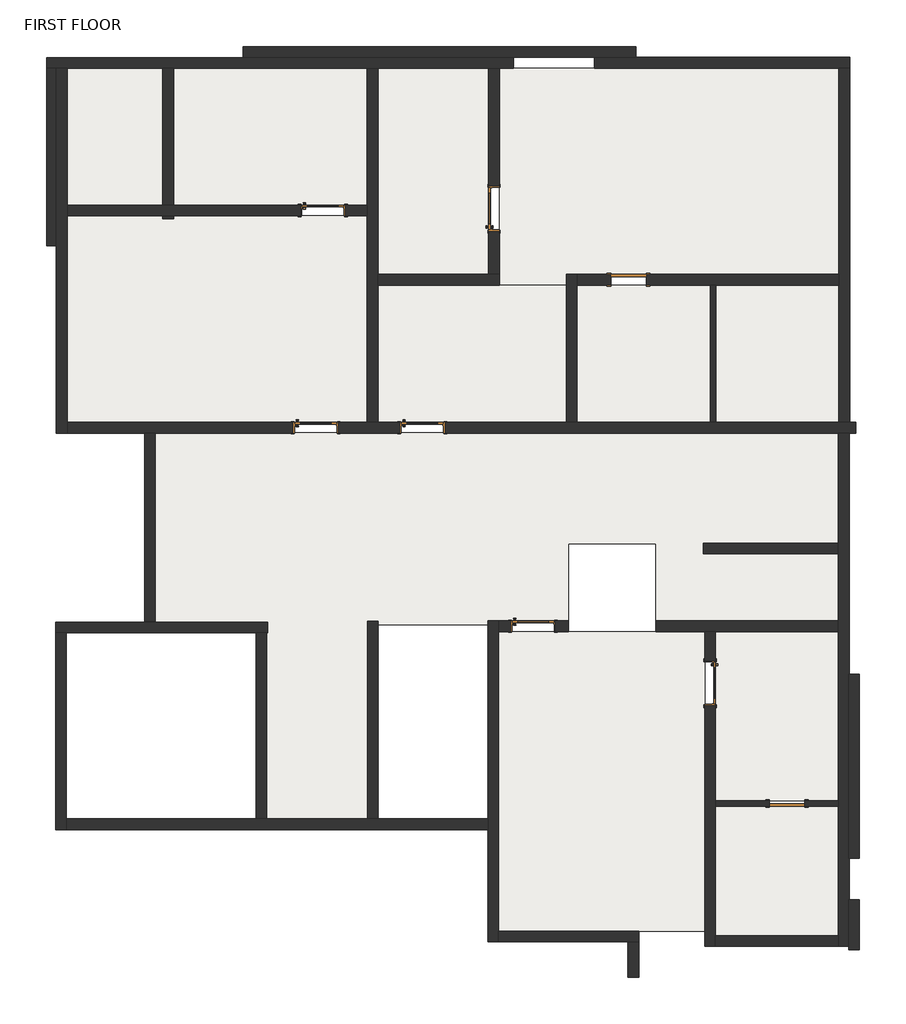
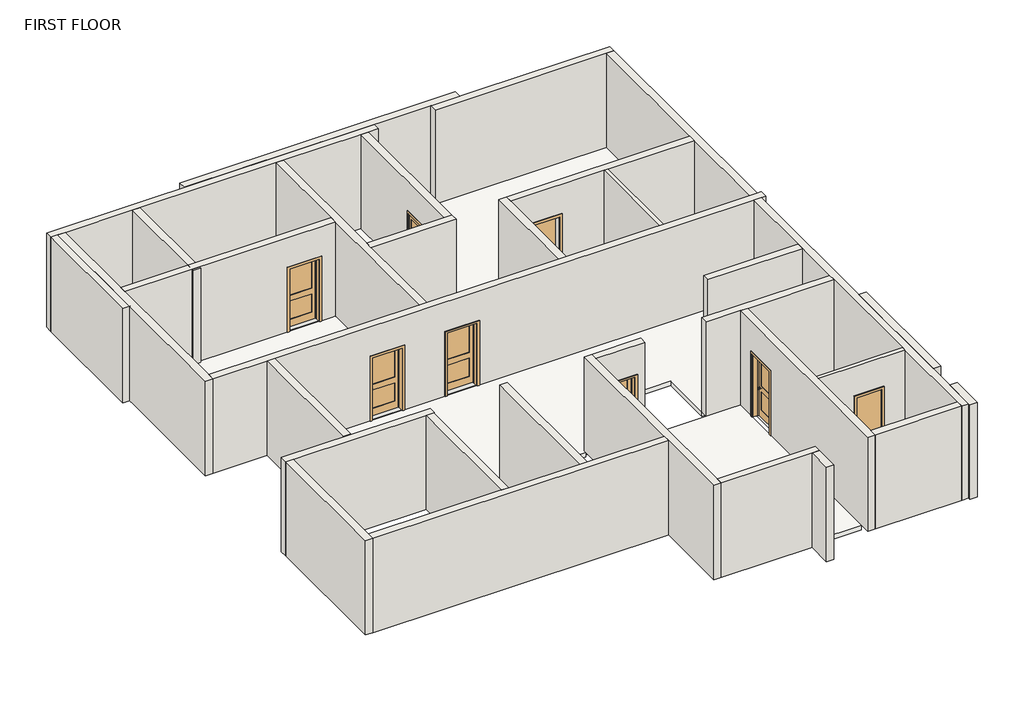
# One storey: 33 walls, 8 doors, 3 slabs.
"""IFC4 building model written with IfcOpenShell, lengths in millimetres."""

from ifc_helpers import new_model, si_unit, frame, origin, place, context, project, spatial, polyline, outline, extrude, faceted_brep, transform, mapped, element, save
from components import door_18b56f29, door_d8f5dbb5, door_a1484949

model = new_model("IFC4")

# Units and contexts
model_context = context("Model", 3, world=origin())
ifc_project = project(units=[si_unit("LENGTHUNIT", "METRE", prefix="MILLI")], contexts=[model_context])

# Site, building, storey
site = spatial("IfcSite", under=ifc_project)
building = spatial("IfcBuilding", under=site)
storey = spatial("IfcBuildingStorey", under=building, Name="FIRST FLOOR", Elevation=3048.0)

# Doors
placement = place(None, origin())
door_shape = door_18b56f29(model_context)
element("IfcDoor", 1, ObjectType="Door-Interior-Single-2_Panel-Wood : 36\" x 80\"", at=placement, inside=storey, context=model_context, shape_type="MappedRepresentation", body=[
    mapped(door_shape, transform((4633.8367729, 4367.107458, 3048.0), x_axis=(1.0, 0.0, 0.0), y_axis=(0.0, 1.0, 0.0), z_axis=(0.0, 0.0, 1.0))),
])
element("IfcDoor", 2, ObjectType="Door-Interior-Single-2_Panel-Wood : 36\" x 80\"", at=placement, inside=storey, context=model_context, shape_type="MappedRepresentation", body=[
    mapped(door_shape, transform((2258.0068953, 8623.6106247, 3048.0), x_axis=(1.0, 0.0, 0.0), y_axis=(0.0, 1.0, 0.0), z_axis=(0.0, 0.0, 1.0))),
])
element("IfcDoor", 3, ObjectType="Door-Interior-Single-2_Panel-Wood : 36\" x 80\"", at=placement, inside=storey, context=model_context, shape_type="MappedRepresentation", body=[
    mapped(door_shape, transform((-27.9931047, 8623.6106247, 3048.0), x_axis=(1.0, 0.0, 0.0), y_axis=(0.0, 1.0, 0.0), z_axis=(0.0, 0.0, 1.0))),
])
element("IfcDoor", 4, ObjectType="Door-Interior-Single-2_Panel-Wood : 36\" x 80\"", at=placement, inside=storey, context=model_context, shape_type="MappedRepresentation", body=[
    mapped(door_shape, transform((124.4068953, 13281.8847639, 3048.0), x_axis=(1.0, 0.0, 0.0), y_axis=(0.0, 1.0, 0.0), z_axis=(0.0, 0.0, 1.0))),
])
element("IfcDoor", 5, ObjectType="Door-Interior-Single-2_Panel-Wood : 36\" x 80\"", at=placement, inside=storey, context=model_context, shape_type="MappedRepresentation", body=[
    mapped(door_shape, transform((3792.558965, 13317.69348, 3048.0), x_axis=(0.0, 1.0, 0.0), y_axis=(-1.0, 0.0, 0.0), z_axis=(0.0, 0.0, 1.0))),
])
element("IfcDoor", 6, ObjectType="Door-Interior-Single-2_Panel-Wood : 36\" x 80\"", at=placement, inside=storey, context=model_context, shape_type="MappedRepresentation", body=[
    mapped(door_shape, transform((8433.5612453, 3144.732458, 3048.0), x_axis=(0.0, -1.0, 0.0), y_axis=(1.0, 0.0, 0.0), z_axis=(0.0, 0.0, 1.0))),
])
door_2_shape = door_d8f5dbb5(model_context)
element("IfcDoor", 7, ObjectType="Single-Flush : 30\" x 80\"", at=placement, inside=storey, context=model_context, shape_type="MappedRepresentation", body=[
    mapped(door_2_shape, transform((10080.5141504, 561.592156, 3048.0), x_axis=(-1.0, 0.0, 0.0), y_axis=(0.0, -1.0, 0.0), z_axis=(0.0, 0.0, 1.0))),
])
door_3_shape = door_a1484949(model_context)
element("IfcDoor", 8, ObjectType="Single-Flush : 30\" x 80\"", at=placement, inside=storey, context=model_context, shape_type="MappedRepresentation", body=[
    mapped(door_3_shape, transform((6680.3464182, 11793.69348, 3048.0), x_axis=(1.0, 0.0, 0.0), y_axis=(0.0, 1.0, 0.0), z_axis=(0.0, 0.0, 1.0))),
])

# Slabs
element("IfcSlab", 9, ObjectType="MARBLE FLOORING 6\"", at=placement, inside=storey, context=model_context, shape_type="SweptSolid", body=[
    extrude(outline(polyline([(-3306.644009, 16327.59348), (-3306.644009, 13393.0097639), (-5364.044009, 13393.0097639), (-5364.044009, 16327.59348), (-3306.644009, 16327.59348)])), frame((0.0, 0.0, 2895.6), z_axis=(0.0, 0.0, 1.0), x_axis=(1.0, 0.0, 0.0)), (0.0, 0.0, 1.0), 152.4),
    extrude(outline(polyline([(1076.9068953, 16327.59348), (1076.9068953, 13393.0097639), (-3078.044009, 13393.0097639), (-3078.044009, 16327.59348), (1076.9068953, 16327.59348)])), frame((0.0, 0.0, 2895.6), z_axis=(0.0, 0.0, 1.0), x_axis=(1.0, 0.0, 0.0)), (0.0, 0.0, 1.0), 152.4),
    extrude(outline(polyline([(3681.433965, 16327.59348), (3681.433965, 11907.99348), (1297.105991, 11907.99348), (1297.105991, 16327.59348), (3681.433965, 16327.59348)])), frame((0.0, 0.0, 2895.6), z_axis=(0.0, 0.0, 1.0), x_axis=(1.0, 0.0, 0.0)), (0.0, 0.0, 1.0), 152.4),
])
element("IfcSlab", 10, ObjectType="MARBLE FLOORING 6\"", at=placement, inside=storey, context=model_context, shape_type="SweptSolid", body=[
    extrude(outline(polyline([(1076.9068953, 13164.4097639), (1076.9068953, 8734.7356247), (-5364.044009, 8734.7356247), (-5364.044009, 13164.4097639), (1076.9068953, 13164.4097639)])), frame((0.0, 0.0, 2895.6), z_axis=(0.0, 0.0, 1.0), x_axis=(1.0, 0.0, 0.0)), (0.0, 0.0, 1.0), 152.4),
    extrude(outline(polyline([(5346.8464182, 11679.39348), (5346.8464182, 8734.7356247), (1305.5068953, 8734.7356247), (1305.5068953, 11679.39348), (5346.8464182, 11679.39348)])), frame((0.0, 0.0, 2895.6), z_axis=(0.0, 0.0, 1.0), x_axis=(1.0, 0.0, 0.0)), (0.0, 0.0, 1.0), 152.4),
])
element("IfcSlab", 11, ObjectType="MARBLE FLOORING 6\"", at=placement, inside=storey, context=model_context, shape_type="SweptSolid", body=[
    extrude(outline(polyline([(8440.081677, 11679.39348), (8440.081677, 8737.3195632), (5575.4464182, 8737.3195632), (5575.4464182, 11679.39348), (8440.081677, 11679.39348)])), frame((0.0, 0.0, 2895.6), z_axis=(0.0, 0.0, 1.0), x_axis=(1.0, 0.0, 0.0)), (0.0, 0.0, 1.0), 152.4),
    extrude(outline(polyline([(11195.981677, 11679.39348), (11195.981677, 8734.7356247), (8554.381677, 8734.7356247), (8554.381677, 11679.39348), (11195.981677, 11679.39348)])), frame((0.0, 0.0, 2895.6), z_axis=(0.0, 0.0, 1.0), x_axis=(1.0, 0.0, 0.0)), (0.0, 0.0, 1.0), 152.4),
    extrude(outline(polyline([(3910.033965, 11679.39348), (3910.033965, 16330.2375339), (11195.981677, 16330.2375339), (11195.981677, 11907.99348), (5346.8464182, 11907.99348), (5346.8464182, 11679.39348), (3910.033965, 11679.39348)])), frame((0.0, 0.0, 2895.6), z_axis=(0.0, 0.0, 1.0), x_axis=(1.0, 0.0, 0.0)), (0.0, 0.0, 1.0), 152.4),
    extrude(outline(polyline([(-3471.744009, 4450.8216143), (-3471.744009, 8508.7195632), (11198.9862453, 8508.7195632), (11198.9862453, 6146.76982), (8289.8141504, 6146.76982), (8289.8141504, 5918.16982), (11185.4141504, 5918.16982), (11185.4141504, 4478.232458), (7273.8141504, 4478.232458), (7273.8141504, 6129.232458), (5395.8367729, 6129.232458), (5395.8367729, 4478.232458), (3668.6367729, 4478.232458), (3668.6367729, 4400.0216143), (1309.2237558, 4400.0216143), (1309.2237558, 4476.2216143), (1080.6237558, 4476.2216143), (1080.6237558, 234.4216143), (-1082.0931047, 234.4216143), (-1082.0931047, 4222.2216143), (-1059.3262442, 4222.2216143), (-1059.3262442, 4450.8216143), (-3471.744009, 4450.8216143)])), frame((0.0, 0.0, 2895.6), z_axis=(0.0, 0.0, 1.0), x_axis=(1.0, 0.0, 0.0)), (0.0, 0.0, 1.0), 152.4),
    extrude(outline(polyline([(8316.0862453, -2170.217542), (3897.2367729, -2170.217542), (3897.2367729, 4249.632458), (8316.0862453, 4249.632458), (8316.0862453, -2170.217542)])), frame((0.0, 0.0, 2895.6), z_axis=(0.0, 0.0, 1.0), x_axis=(1.0, 0.0, 0.0)), (0.0, 0.0, 1.0), 152.4),
    extrude(outline(polyline([(8544.6862453, 618.742156), (8544.6862453, 4249.632458), (11185.4141504, 4249.632458), (11185.4141504, 618.742156), (8544.6862453, 618.742156)])), frame((0.0, 0.0, 2895.6), z_axis=(0.0, 0.0, 1.0), x_axis=(1.0, 0.0, 0.0)), (0.0, 0.0, 1.0), 152.4),
    extrude(outline(polyline([(8544.6862453, -2271.817542), (8544.6862453, 504.442156), (11185.4141504, 504.442156), (11185.4141504, -2271.817542), (8544.6862453, -2271.817542)])), frame((0.0, 0.0, 2895.6), z_axis=(0.0, 0.0, 1.0), x_axis=(1.0, 0.0, 0.0)), (0.0, 0.0, 1.0), 152.4),
])

# Walls
element("IfcWall", 12, ObjectType="INNER WALL 4.5\"", at=placement, inside=storey, context=model_context, shape_type="SweptSolid", body=[
    extrude(outline(polyline([(3048.0, 8544.6862453), (3048.0, 9699.5141504), (5080.0, 9699.5141504), (5080.0, 10461.5141504), (3048.0, 10461.5141504), (3048.0, 11185.4141504), (6096.0, 11185.4141504), (6096.0, 8544.6862453), (3048.0, 8544.6862453)])), frame((0.0, 504.442156, 0.0), z_axis=(0.0, 1.0, 0.0), x_axis=(0.0, 0.0, 1.0)), (0.0, 0.0, 1.0), 114.3),
])
element("IfcWall", 13, ObjectType="INNER WALL 4.5\"", at=placement, inside=storey, context=model_context, shape_type="SweptSolid", body=[
    extrude(outline(polyline([(8440.081677, 8737.3195632), (8440.081677, 11679.39348), (8554.381677, 11679.39348), (8554.381677, 8737.3195632), (8440.081677, 8737.3195632)])), frame((0.0, 0.0, 3048.0), z_axis=(0.0, 0.0, 1.0), x_axis=(1.0, 0.0, 0.0)), (0.0, 0.0, 1.0), 3048.0),
])
element("IfcWall", 14, ObjectType="OUTER WALL THICKNESS 9\"", at=placement, inside=storey, context=model_context, shape_type="Brep", body=[
    faceted_brep([(11424.581677, 16558.8375339, 3048.0), (5950.881677, 16558.8375339, 3048.0), (5950.881677, 16558.8375339, 6096.0), (11424.581677, 16558.8375339, 6096.0), (11424.581677, 16330.2375339, 3048.0), (11424.581677, 16330.2375339, 6096.0), (11195.981677, 16330.2375339, 6096.0), (5950.881677, 16330.2375339, 6096.0), (5950.881677, 16330.2375339, 3048.0), (11195.981677, 16330.2375339, 3048.0)], [[[0, 1, 2, 3]], [[4, 5, 6, 7, 8, 9]], [[1, 0, 4, 9, 8]], [[2, 1, 8, 7]], [[3, 2, 7, 6, 5]], [[0, 3, 5, 4]]]),
])
element("IfcWall", 15, ObjectType="OUTER WALL THICKNESS 9\"", at=placement, inside=storey, context=model_context, shape_type="SweptSolid", body=[
    extrude(outline(polyline([(-1588.9187543, 16792.7871664), (6843.8812457, 16792.7871664), (6843.8812457, 16564.1871664), (-1588.9187543, 16564.1871664), (-1588.9187543, 16792.7871664)])), frame((0.0, 0.0, 3048.0), z_axis=(0.0, 0.0, 1.0), x_axis=(1.0, 0.0, 0.0)), (0.0, 0.0, 1.0), 3048.0),
])
element("IfcWall", 16, ObjectType="OUTER WALL THICKNESS 9\"", at=placement, inside=storey, context=model_context, shape_type="Brep", body=[
    faceted_brep([(4217.331677, 16556.19348, 3048.0), (-5802.968323, 16556.19348, 3048.0), (-5802.968323, 16556.19348, 6096.0), (4217.331677, 16556.19348, 6096.0), (4217.331677, 16327.59348, 3048.0), (4217.331677, 16327.59348, 6096.0), (3910.033965, 16327.59348, 6096.0), (3681.433965, 16327.59348, 6096.0), (1305.5068953, 16327.59348, 6096.0), (1076.9068953, 16327.59348, 6096.0), (-3078.044009, 16327.59348, 6096.0), (-3306.644009, 16327.59348, 6096.0), (-5364.044009, 16327.59348, 6096.0), (-5574.368323, 16327.59348, 6096.0), (-5592.644009, 16327.59348, 6096.0), (-5802.968323, 16327.59348, 6096.0), (-5802.968323, 16327.59348, 3048.0), (-5592.644009, 16327.59348, 3048.0), (-5574.368323, 16327.59348, 3048.0), (-5364.044009, 16327.59348, 3048.0), (-3306.644009, 16327.59348, 3048.0), (-3078.044009, 16327.59348, 3048.0), (1076.9068953, 16327.59348, 3048.0), (1305.5068953, 16327.59348, 3048.0), (3681.433965, 16327.59348, 3048.0), (3910.033965, 16327.59348, 3048.0)], [[[0, 1, 2, 3]], [[4, 5, 6, 7, 8, 9, 10, 11, 12, 13, 14, 15, 16, 17, 18, 19, 20, 21, 22, 23, 24, 25]], [[1, 0, 4, 25, 24, 23, 22, 21, 20, 19, 18, 17, 16]], [[3, 2, 15, 14, 13, 12, 11, 10, 9, 8, 7, 6, 5]], [[0, 3, 5, 4]], [[2, 1, 16, 15]]]),
])
element("IfcWall", 17, ObjectType="OUTER WALL THICKNESS 9\"", at=placement, inside=storey, context=model_context, shape_type="SweptSolid", body=[
    extrude(outline(polyline([(-5802.968323, 12517.59348), (-5802.968323, 16327.59348), (-5574.368323, 16327.59348), (-5574.368323, 12517.59348), (-5802.968323, 12517.59348)])), frame((0.0, 0.0, 3048.0), z_axis=(0.0, 0.0, 1.0), x_axis=(1.0, 0.0, 0.0)), (0.0, 0.0, 1.0), 3048.0),
])
element("IfcWall", 18, ObjectType="OUTER WALL THICKNESS 9\"", at=placement, inside=storey, context=model_context, shape_type="Brep", body=[
    faceted_brep([(-5364.044009, 8504.39348, 3048.0), (-5364.044009, 8506.1356247, 3048.0), (-5364.044009, 8734.7356247, 3048.0), (-5364.044009, 13164.4097639, 3048.0), (-5364.044009, 13393.0097639, 3048.0), (-5364.044009, 16327.59348, 3048.0), (-5364.044009, 16327.59348, 6096.0), (-5364.044009, 13393.0097639, 6096.0), (-5364.044009, 13164.4097639, 6096.0), (-5364.044009, 8734.7356247, 6096.0), (-5364.044009, 8506.1356247, 6096.0), (-5364.044009, 8504.39348, 6096.0), (-5592.644009, 8504.39348, 3048.0), (-5592.644009, 8504.39348, 6096.0), (-5592.644009, 16327.59348, 6096.0), (-5592.644009, 16327.59348, 3048.0)], [[[0, 1, 2, 3, 4, 5, 6, 7, 8, 9, 10, 11]], [[12, 13, 14, 15]], [[5, 4, 3, 2, 1, 0, 12, 15]], [[11, 10, 9, 8, 7, 6, 14, 13]], [[0, 11, 13, 12]], [[6, 5, 15, 14]]]),
])
element("IfcWall", 19, ObjectType="OUTER WALL THICKNESS 9\"", at=placement, inside=storey, context=model_context, shape_type="Brep", body=[
    faceted_brep([(11552.355991, 8506.1356247, 3048.0), (11552.355991, 8506.1356247, 6096.0), (11414.0141504, 8506.1356247, 6096.0), (11185.4141504, 8506.1356247, 6096.0), (-5364.044009, 8506.1356247, 6096.0), (-5364.044009, 8506.1356247, 3048.0), (-510.5931047, 8506.1356247, 3048.0), (-510.5931047, 8506.1356247, 5105.4), (454.6068953, 8506.1356247, 5105.4), (454.6068953, 8506.1356247, 3048.0), (1775.4068953, 8506.1356247, 3048.0), (1775.4068953, 8506.1356247, 5105.4), (2740.6068953, 8506.1356247, 5105.4), (2740.6068953, 8506.1356247, 3048.0), (11185.4141504, 8506.1356247, 3048.0), (11414.0141504, 8506.1356247, 3048.0), (11552.355991, 8734.7356247, 6096.0), (11552.355991, 8734.7356247, 3048.0), (11424.581677, 8734.7356247, 3048.0), (11195.981677, 8734.7356247, 3048.0), (5575.4464182, 8734.7356247, 3048.0), (5346.8464182, 8734.7356247, 3048.0), (2740.6068953, 8734.7356247, 3048.0), (2740.6068953, 8734.7356247, 5105.4), (1775.4068953, 8734.7356247, 5105.4), (1775.4068953, 8734.7356247, 3048.0), (1305.5068953, 8734.7356247, 3048.0), (1076.9068953, 8734.7356247, 3048.0), (454.6068953, 8734.7356247, 3048.0), (454.6068953, 8734.7356247, 5105.4), (-510.5931047, 8734.7356247, 5105.4), (-510.5931047, 8734.7356247, 3048.0), (-5364.044009, 8734.7356247, 3048.0), (-5364.044009, 8734.7356247, 6096.0), (1076.9068953, 8734.7356247, 6096.0), (1305.5068953, 8734.7356247, 6096.0), (5346.8464182, 8734.7356247, 6096.0), (5575.4464182, 8734.7356247, 6096.0), (11195.981677, 8734.7356247, 6096.0), (11424.581677, 8734.7356247, 6096.0)], [[[0, 1, 2, 3, 4, 5, 6, 7, 8, 9, 10, 11, 12, 13, 14, 15]], [[16, 17, 18, 19, 20, 21, 22, 23, 24, 25, 26, 27, 28, 29, 30, 31, 32, 33, 34, 35, 36, 37, 38, 39]], [[17, 0, 15, 14, 13, 22, 21, 20, 19, 18]], [[5, 32, 31, 6]], [[25, 10, 9, 28, 27, 26]], [[1, 0, 17, 16]], [[4, 3, 2, 1, 16, 39, 38, 37, 36, 35, 34, 33]], [[5, 4, 33, 32]], [[12, 23, 22, 13]], [[23, 12, 11, 24]], [[24, 11, 10, 25]], [[8, 29, 28, 9]], [[29, 8, 7, 30]], [[30, 7, 6, 31]]]),
])
element("IfcWall", 20, ObjectType="OUTER WALL THICKNESS 9\"", at=placement, inside=storey, context=model_context, shape_type="Brep", body=[
    faceted_brep([(5575.4464182, 8734.7356247, 3048.0), (5575.4464182, 11679.39348, 3048.0), (5575.4464182, 11907.99348, 3048.0), (5575.4464182, 11907.99348, 6096.0), (5575.4464182, 11679.39348, 6096.0), (5575.4464182, 8734.7356247, 6096.0), (5346.8464182, 8734.7356247, 3048.0), (5346.8464182, 8734.7356247, 6096.0), (5346.8464182, 11907.99348, 6096.0), (5346.8464182, 11907.99348, 3048.0)], [[[0, 1, 2, 3, 4, 5]], [[6, 7, 8, 9]], [[2, 1, 0, 6, 9]], [[5, 4, 3, 8, 7]], [[0, 5, 7, 6]], [[3, 2, 9, 8]]]),
])
element("IfcWall", 21, ObjectType="OUTER WALL THICKNESS 9\"", at=placement, inside=storey, context=model_context, shape_type="Brep", body=[
    faceted_brep([(1305.5068953, 8734.7356247, 3048.0), (1305.5068953, 11679.39348, 3048.0), (1305.5068953, 11907.99348, 3048.0), (1305.5068953, 16327.59348, 3048.0), (1305.5068953, 16327.59348, 6096.0), (1305.5068953, 11907.99348, 6096.0), (1305.5068953, 11679.39348, 6096.0), (1305.5068953, 8734.7356247, 6096.0), (1076.9068953, 8734.7356247, 3048.0), (1076.9068953, 8734.7356247, 6096.0), (1076.9068953, 13164.4097639, 6096.0), (1076.9068953, 13393.0097639, 6096.0), (1076.9068953, 16327.59348, 6096.0), (1076.9068953, 16327.59348, 3048.0), (1076.9068953, 13393.0097639, 3048.0), (1076.9068953, 13164.4097639, 3048.0)], [[[0, 1, 2, 3, 4, 5, 6, 7]], [[8, 9, 10, 11, 12, 13, 14, 15]], [[3, 2, 1, 0, 8, 15, 14, 13]], [[7, 6, 5, 4, 12, 11, 10, 9]], [[4, 3, 13, 12]], [[0, 7, 9, 8]]]),
])
element("IfcWall", 22, ObjectType="OUTER WALL THICKNESS 9\"", at=placement, inside=storey, context=model_context, shape_type="SweptSolid", body=[
    extrude(outline(polyline([(-3306.644009, 13101.79348), (-3306.644009, 16327.59348), (-3078.044009, 16327.59348), (-3078.044009, 13101.79348), (-3306.644009, 13101.79348)])), frame((0.0, 0.0, 3048.0), z_axis=(0.0, 0.0, 1.0), x_axis=(1.0, 0.0, 0.0)), (0.0, 0.0, 1.0), 3048.0),
])
element("IfcWall", 23, ObjectType="OUTER WALL THICKNESS 9\"", at=placement, inside=storey, context=model_context, shape_type="SweptSolid", body=[
    extrude(outline(polyline([(6096.0, 1076.9068953), (6096.0, -5364.044009), (3048.0, -5364.044009), (3048.0, -358.1931047), (5105.4, -358.1931047), (5105.4, 607.0068953), (3048.0, 607.0068953), (3048.0, 1076.9068953), (6096.0, 1076.9068953)])), frame((0.0, 13164.4097639, 0.0), z_axis=(0.0, 1.0, 0.0), x_axis=(0.0, 0.0, 1.0)), (0.0, 0.0, 1.0), 228.6),
])
element("IfcWall", 24, ObjectType="OUTER WALL THICKNESS 9\"", at=placement, inside=storey, context=model_context, shape_type="Brep", body=[
    faceted_brep([(1305.5068953, 11679.39348, 3048.0), (3910.033965, 11679.39348, 3048.0), (3910.033965, 11679.39348, 6096.0), (1305.5068953, 11679.39348, 6096.0), (1305.5068953, 11907.99348, 3048.0), (1305.5068953, 11907.99348, 6096.0), (3681.433965, 11907.99348, 6096.0), (3910.033965, 11907.99348, 6096.0), (3910.033965, 11907.99348, 3048.0), (3681.433965, 11907.99348, 3048.0)], [[[0, 1, 2, 3]], [[4, 5, 6, 7, 8, 9]], [[1, 0, 4, 9, 8]], [[3, 2, 7, 6, 5]], [[0, 3, 5, 4]], [[2, 1, 8, 7]]]),
])
element("IfcWall", 25, ObjectType="OUTER WALL THICKNESS 9\"", at=placement, inside=storey, context=model_context, shape_type="SweptSolid", body=[
    extrude(outline(polyline([(11907.99348, 6096.0), (16327.59348, 6096.0), (16327.59348, 3048.0), (13800.29348, 3048.0), (13800.29348, 5105.4), (12835.09348, 5105.4), (12835.09348, 3048.0), (11907.99348, 3048.0), (11907.99348, 6096.0)])), frame((3681.433965, 0.0, 0.0), z_axis=(1.0, 0.0, 0.0), x_axis=(0.0, 1.0, 0.0)), (0.0, 0.0, 1.0), 228.6),
])
element("IfcWall", 26, ObjectType="OUTER WALL THICKNESS 9\"", at=placement, inside=storey, context=model_context, shape_type="Brep", body=[
    faceted_brep([(11414.0141504, -2500.417542, 3048.0), (11414.0141504, 8506.1356247, 3048.0), (11414.0141504, 8506.1356247, 6096.0), (11414.0141504, -2500.417542, 6096.0), (11185.4141504, -2500.417542, 3048.0), (11185.4141504, -2500.417542, 6096.0), (11185.4141504, -2271.817542, 6096.0), (11185.4141504, 504.442156, 6096.0), (11185.4141504, 618.742156, 6096.0), (11185.4141504, 4249.632458, 6096.0), (11185.4141504, 4478.232458, 6096.0), (11185.4141504, 5918.16982, 6096.0), (11185.4141504, 6146.76982, 6096.0), (11185.4141504, 8506.1356247, 6096.0), (11185.4141504, 8506.1356247, 3048.0), (11185.4141504, 6146.76982, 3048.0), (11185.4141504, 5918.16982, 3048.0), (11185.4141504, 4478.232458, 3048.0), (11185.4141504, 4249.632458, 3048.0), (11185.4141504, 618.742156, 3048.0), (11185.4141504, 504.442156, 3048.0), (11185.4141504, -2271.817542, 3048.0)], [[[0, 1, 2, 3]], [[4, 5, 6, 7, 8, 9, 10, 11, 12, 13, 14, 15, 16, 17, 18, 19, 20, 21]], [[1, 0, 4, 21, 20, 19, 18, 17, 16, 15, 14]], [[3, 2, 13, 12, 11, 10, 9, 8, 7, 6, 5]], [[2, 1, 14, 13]], [[0, 3, 5, 4]]]),
])
element("IfcWall", 27, ObjectType="OUTER WALL THICKNESS 9\"", at=placement, inside=storey, context=model_context, shape_type="Brep", body=[
    faceted_brep([(-5605.9262442, 4222.2216143, 3048.0), (-5377.3262442, 4222.2216143, 3048.0), (-1310.6931047, 4222.2216143, 3048.0), (-1082.0931047, 4222.2216143, 3048.0), (-1059.3262442, 4222.2216143, 3048.0), (-1059.3262442, 4222.2216143, 6096.0), (-1082.0931047, 4222.2216143, 6096.0), (-1310.6931047, 4222.2216143, 6096.0), (-5377.3262442, 4222.2216143, 6096.0), (-5605.9262442, 4222.2216143, 6096.0), (-5605.9262442, 4450.8216143, 3048.0), (-5605.9262442, 4450.8216143, 6096.0), (-1059.3262442, 4450.8216143, 6096.0), (-1059.3262442, 4450.8216143, 3048.0)], [[[0, 1, 2, 3, 4, 5, 6, 7, 8, 9]], [[10, 11, 12, 13]], [[4, 3, 2, 1, 0, 10, 13]], [[5, 4, 13, 12]], [[9, 8, 7, 6, 5, 12, 11]], [[0, 9, 11, 10]]]),
])
element("IfcWall", 28, ObjectType="OUTER WALL THICKNESS 9\"", at=placement, inside=storey, context=model_context, shape_type="SweptSolid", body=[
    extrude(outline(polyline([(-3700.344009, 4476.2216143), (-3700.344009, 8504.39348), (-3471.744009, 8504.39348), (-3471.744009, 4476.2216143), (-3700.344009, 4476.2216143)])), frame((0.0, 0.0, 3048.0), z_axis=(0.0, 0.0, 1.0), x_axis=(1.0, 0.0, 0.0)), (0.0, 0.0, 1.0), 3048.0),
])
element("IfcWall", 29, ObjectType="OUTER WALL THICKNESS 9\"", at=placement, inside=storey, context=model_context, shape_type="Brep", body=[
    faceted_brep([(-5605.9262442, 4222.2216143, 3048.0), (-5605.9262442, 5.8216143, 3048.0), (-5605.9262442, 5.8216143, 6096.0), (-5605.9262442, 4222.2216143, 6096.0), (-5377.3262442, 4222.2216143, 3048.0), (-5377.3262442, 4222.2216143, 6096.0), (-5377.3262442, 234.4216143, 6096.0), (-5377.3262442, 5.8216143, 6096.0), (-5377.3262442, 5.8216143, 3048.0), (-5377.3262442, 234.4216143, 3048.0)], [[[0, 1, 2, 3]], [[4, 5, 6, 7, 8, 9]], [[1, 0, 4, 9, 8]], [[3, 2, 7, 6, 5]], [[0, 3, 5, 4]], [[2, 1, 8, 7]]]),
])
element("IfcWall", 30, ObjectType="OUTER WALL THICKNESS 9\"", at=placement, inside=storey, context=model_context, shape_type="Brep", body=[
    faceted_brep([(3668.6367729, 234.4216143, 3048.0), (1309.2237558, 234.4216143, 3048.0), (1080.6237558, 234.4216143, 3048.0), (-1082.0931047, 234.4216143, 3048.0), (-1310.6931047, 234.4216143, 3048.0), (-5377.3262442, 234.4216143, 3048.0), (-5377.3262442, 234.4216143, 6096.0), (-1310.6931047, 234.4216143, 6096.0), (-1082.0931047, 234.4216143, 6096.0), (1080.6237558, 234.4216143, 6096.0), (1309.2237558, 234.4216143, 6096.0), (3668.6367729, 234.4216143, 6096.0), (3668.6367729, 5.8216143, 3048.0), (3668.6367729, 5.8216143, 6096.0), (-5377.3262442, 5.8216143, 6096.0), (-5377.3262442, 5.8216143, 3048.0)], [[[0, 1, 2, 3, 4, 5, 6, 7, 8, 9, 10, 11]], [[12, 13, 14, 15]], [[5, 4, 3, 2, 1, 0, 12, 15]], [[11, 10, 9, 8, 7, 6, 14, 13]], [[6, 5, 15, 14]], [[0, 11, 13, 12]]]),
])
element("IfcWall", 31, ObjectType="OUTER WALL THICKNESS 9\"", at=placement, inside=storey, context=model_context, shape_type="SweptSolid", body=[
    extrude(outline(polyline([(-1310.6931047, 234.4216143), (-1310.6931047, 4222.2216143), (-1082.0931047, 4222.2216143), (-1082.0931047, 234.4216143), (-1310.6931047, 234.4216143)])), frame((0.0, 0.0, 3048.0), z_axis=(0.0, 0.0, 1.0), x_axis=(1.0, 0.0, 0.0)), (0.0, 0.0, 1.0), 3048.0),
])
element("IfcWall", 32, ObjectType="OUTER WALL THICKNESS 9\"", at=placement, inside=storey, context=model_context, shape_type="SweptSolid", body=[
    extrude(outline(polyline([(1080.6237558, 234.4216143), (1080.6237558, 4476.2216143), (1309.2237558, 4476.2216143), (1309.2237558, 234.4216143), (1080.6237558, 234.4216143)])), frame((0.0, 0.0, 3048.0), z_axis=(0.0, 0.0, 1.0), x_axis=(1.0, 0.0, 0.0)), (0.0, 0.0, 1.0), 3048.0),
])
element("IfcWall", 33, ObjectType="OUTER WALL THICKNESS 9\"", at=placement, inside=storey, context=model_context, shape_type="SweptSolid", body=[
    extrude(outline(polyline([(8289.8141504, 6146.76982), (11185.4141504, 6146.76982), (11185.4141504, 5918.16982), (8289.8141504, 5918.16982), (8289.8141504, 6146.76982)])), frame((0.0, 0.0, 3048.0), z_axis=(0.0, 0.0, 1.0), x_axis=(1.0, 0.0, 0.0)), (0.0, 0.0, 1.0), 3048.0),
])
element("IfcWall", 34, ObjectType="OUTER WALL THICKNESS 9\"", at=placement, inside=storey, context=model_context, shape_type="Brep", body=[
    faceted_brep([(3897.2367729, -2398.817542, 3048.0), (3897.2367729, -2170.217542, 3048.0), (3897.2367729, 4249.632458, 3048.0), (3897.2367729, 4478.232458, 3048.0), (3897.2367729, 4478.232458, 6096.0), (3897.2367729, 4249.632458, 6096.0), (3897.2367729, -2170.217542, 6096.0), (3897.2367729, -2398.817542, 6096.0), (3668.6367729, -2398.817542, 3048.0), (3668.6367729, -2398.817542, 6096.0), (3668.6367729, 5.8216143, 6096.0), (3668.6367729, 234.4216143, 6096.0), (3668.6367729, 4478.232458, 6096.0), (3668.6367729, 4478.232458, 3048.0), (3668.6367729, 234.4216143, 3048.0), (3668.6367729, 5.8216143, 3048.0)], [[[0, 1, 2, 3, 4, 5, 6, 7]], [[8, 9, 10, 11, 12, 13, 14, 15]], [[3, 2, 1, 0, 8, 15, 14, 13]], [[7, 6, 5, 4, 12, 11, 10, 9]], [[4, 3, 13, 12]], [[0, 7, 9, 8]]]),
])
element("IfcWall", 35, ObjectType="OUTER WALL THICKNESS 9\"", at=placement, inside=storey, context=model_context, shape_type="SweptSolid", body=[
    extrude(outline(polyline([(3048.0, 5395.8367729), (6096.0, 5395.8367729), (6096.0, 3897.2367729), (3048.0, 3897.2367729), (3048.0, 4151.2367729), (5105.4, 4151.2367729), (5105.4, 5116.4367729), (3048.0, 5116.4367729), (3048.0, 5395.8367729)])), frame((0.0, 4249.632458, 0.0), z_axis=(0.0, 1.0, 0.0), x_axis=(0.0, 0.0, 1.0)), (0.0, 0.0, 1.0), 228.6),
])
element("IfcWall", 36, ObjectType="OUTER WALL THICKNESS 9\"", at=placement, inside=storey, context=model_context, shape_type="Brep", body=[
    faceted_brep([(3897.2367729, -2398.817542, 3048.0), (6670.8415275, -2398.817542, 3048.0), (6899.4415275, -2398.817542, 3048.0), (6899.4415275, -2398.817542, 6096.0), (6670.8415275, -2398.817542, 6096.0), (3897.2367729, -2398.817542, 6096.0), (3897.2367729, -2170.217542, 3048.0), (3897.2367729, -2170.217542, 6096.0), (6899.4415275, -2170.217542, 6096.0), (6899.4415275, -2170.217542, 3048.0)], [[[0, 1, 2, 3, 4, 5]], [[6, 7, 8, 9]], [[2, 1, 0, 6, 9]], [[5, 4, 3, 8, 7]], [[0, 5, 7, 6]], [[3, 2, 9, 8]]]),
])
element("IfcWall", 37, ObjectType="OUTER WALL THICKNESS 9\"", at=placement, inside=storey, context=model_context, shape_type="SweptSolid", body=[
    extrude(outline(polyline([(6899.4415275, -2398.817542), (6899.4415275, -3165.0421945), (6670.8415275, -3165.0421945), (6670.8415275, -2398.817542), (6899.4415275, -2398.817542)])), frame((0.0, 0.0, 3048.0), z_axis=(0.0, 0.0, 1.0), x_axis=(1.0, 0.0, 0.0)), (0.0, 0.0, 1.0), 3048.0),
])
element("IfcWall", 38, ObjectType="OUTER WALL THICKNESS 9\"", at=placement, inside=storey, context=model_context, shape_type="SweptSolid", body=[
    extrude(outline(polyline([(11404.575879, -613.5466507), (11404.575879, 3336.0064687), (11633.175879, 3336.0064687), (11633.175879, -613.5466507), (11404.575879, -613.5466507)])), frame((0.0, 0.0, 3048.0), z_axis=(0.0, 0.0, 1.0), x_axis=(1.0, 0.0, 0.0)), (0.0, 0.0, 1.0), 3048.0),
])
element("IfcWall", 39, ObjectType="OUTER WALL THICKNESS 9\"", at=placement, inside=storey, context=model_context, shape_type="SweptSolid", body=[
    extrude(outline(polyline([(11404.575879, -2569.3466507), (11404.575879, -1502.5466507), (11633.175879, -1502.5466507), (11633.175879, -2569.3466507), (11404.575879, -2569.3466507)])), frame((0.0, 0.0, 3048.0), z_axis=(0.0, 0.0, 1.0), x_axis=(1.0, 0.0, 0.0)), (0.0, 0.0, 1.0), 3048.0),
])
element("IfcWall", 40, ObjectType="OUTER WALL THICKNESS 9\"", at=placement, inside=storey, context=model_context, shape_type="Brep", body=[
    faceted_brep([(11185.4141504, 4478.232458, 3048.0), (7273.8141504, 4478.232458, 3048.0), (7273.8141504, 4478.232458, 6096.0), (11185.4141504, 4478.232458, 6096.0), (11185.4141504, 4249.632458, 3048.0), (11185.4141504, 4249.632458, 6096.0), (8544.6862453, 4249.632458, 6096.0), (8316.0862453, 4249.632458, 6096.0), (7273.8141504, 4249.632458, 6096.0), (7273.8141504, 4249.632458, 3048.0), (8316.0862453, 4249.632458, 3048.0), (8544.6862453, 4249.632458, 3048.0)], [[[0, 1, 2, 3]], [[4, 5, 6, 7, 8, 9, 10, 11]], [[1, 0, 4, 11, 10, 9]], [[2, 1, 9, 8]], [[3, 2, 8, 7, 6, 5]], [[0, 3, 5, 4]]]),
])
element("IfcWall", 41, ObjectType="OUTER WALL THICKNESS 9\"", at=placement, inside=storey, context=model_context, shape_type="Brep", body=[
    faceted_brep([(8316.0862453, -2500.417542, 6096.0), (8316.0862453, 4249.632458, 6096.0), (8316.0862453, 4249.632458, 3048.0), (8316.0862453, 3627.332458, 3048.0), (8316.0862453, 3627.332458, 5105.4), (8316.0862453, 2662.132458, 5105.4), (8316.0862453, 2662.132458, 3048.0), (8316.0862453, -2500.417542, 3048.0), (8544.6862453, 4249.632458, 6096.0), (8544.6862453, 618.742156, 6096.0), (8544.6862453, 504.442156, 6096.0), (8544.6862453, -2271.817542, 6096.0), (8544.6862453, -2500.417542, 6096.0), (8544.6862453, -2500.417542, 3048.0), (8544.6862453, -2271.817542, 3048.0), (8544.6862453, 504.442156, 3048.0), (8544.6862453, 618.742156, 3048.0), (8544.6862453, 2662.132458, 3048.0), (8544.6862453, 2662.132458, 5105.4), (8544.6862453, 3627.332458, 5105.4), (8544.6862453, 3627.332458, 3048.0), (8544.6862453, 4249.632458, 3048.0)], [[[0, 1, 2, 3, 4, 5, 6, 7]], [[8, 9, 10, 11, 12, 13, 14, 15, 16, 17, 18, 19, 20, 21]], [[2, 21, 20, 3]], [[13, 7, 6, 17, 16, 15, 14]], [[1, 0, 12, 11, 10, 9, 8]], [[2, 1, 8, 21]], [[0, 7, 13, 12]], [[5, 18, 17, 6]], [[18, 5, 4, 19]], [[19, 4, 3, 20]]]),
])
element("IfcWall", 42, ObjectType="OUTER WALL THICKNESS 9\"", at=placement, inside=storey, context=model_context, shape_type="SweptSolid", body=[
    extrude(outline(polyline([(11185.4141504, -2500.417542), (8544.6862453, -2500.417542), (8544.6862453, -2271.817542), (11185.4141504, -2271.817542), (11185.4141504, -2500.417542)])), frame((0.0, 0.0, 3048.0), z_axis=(0.0, 0.0, 1.0), x_axis=(1.0, 0.0, 0.0)), (0.0, 0.0, 1.0), 3048.0),
])
element("IfcWall", 43, ObjectType="OUTER WALL THICKNESS 9\"", at=placement, inside=storey, context=model_context, shape_type="Brep", body=[
    faceted_brep([(11195.981677, 16330.2375339, 3048.0), (11195.981677, 11907.99348, 3048.0), (11195.981677, 11679.39348, 3048.0), (11195.981677, 8734.7356247, 3048.0), (11195.981677, 8734.7356247, 6096.0), (11195.981677, 11679.39348, 6096.0), (11195.981677, 11907.99348, 6096.0), (11195.981677, 16330.2375339, 6096.0), (11424.581677, 16330.2375339, 3048.0), (11424.581677, 16330.2375339, 6096.0), (11424.581677, 8734.7356247, 6096.0), (11424.581677, 8734.7356247, 3048.0)], [[[0, 1, 2, 3, 4, 5, 6, 7]], [[8, 9, 10, 11]], [[3, 2, 1, 0, 8, 11]], [[7, 6, 5, 4, 10, 9]], [[0, 7, 9, 8]], [[4, 3, 11, 10]]]),
])
element("IfcWall", 44, ObjectType="OUTER WALL THICKNESS 9\"", at=placement, inside=storey, context=model_context, shape_type="Brep", body=[
    faceted_brep([(7061.3464182, 11679.39348, 5080.0), (7061.3464182, 11679.39348, 3048.0), (8440.081677, 11679.39348, 3048.0), (8554.381677, 11679.39348, 3048.0), (11195.981677, 11679.39348, 3048.0), (11195.981677, 11679.39348, 6096.0), (8554.381677, 11679.39348, 6096.0), (8440.081677, 11679.39348, 6096.0), (5575.4464182, 11679.39348, 6096.0), (5575.4464182, 11679.39348, 3048.0), (6299.3464182, 11679.39348, 3048.0), (6299.3464182, 11679.39348, 5080.0), (11195.981677, 11907.99348, 3048.0), (7061.3464182, 11907.99348, 3048.0), (7061.3464182, 11907.99348, 5080.0), (6299.3464182, 11907.99348, 5080.0), (6299.3464182, 11907.99348, 3048.0), (5575.4464182, 11907.99348, 3048.0), (5575.4464182, 11907.99348, 6096.0), (11195.981677, 11907.99348, 6096.0)], [[[0, 1, 2, 3, 4, 5, 6, 7, 8, 9, 10, 11]], [[12, 13, 14, 15, 16, 17, 18, 19]], [[10, 9, 17, 16]], [[4, 3, 2, 1, 13, 12]], [[8, 7, 6, 5, 19, 18]], [[9, 8, 18, 17]], [[5, 4, 12, 19]], [[14, 13, 1, 0]], [[15, 14, 0, 11]], [[16, 15, 11, 10]]]),
])

save(model, "model.ifc")

# Revit data of these elements
# Type "Door-Interior-Single-2_Panel-Wood : 36\" x 80\""
#   Type Mark = "8"
#   Assembly Code = "C1020300"
#   Analytic Construction = "Wooden"
#   Top Rail = 0' - 4 11/16"
#   Thickness = 0' - 1 3/8"
#   Thermal Resistance (R) = 2.5876 (h·ft²·°F)/BTU
#   Swing Angle [instance default] = 90.00°
#   Stiles = 0' - 4 3/4"
#   Rough Width = 3' - 2"
#   Rough Height = 6' - 9"
#   Lock Rail = 0' - 7 1/2"
#   Height = 6' - 8"
#   Width = 3' - 0"
#   Heat Transfer Coefficient (U) = 0.3865 BTU/(h·ft²·°F)
#   Bottom Rail = 0' - 9 1/8"
#   Trim Material = Cherry
#   Panel Material = Cherry
#   Frame Material = Cherry
#   Door Handle Material = Aluminum
#   Visual Light Transmittance = 0
#   Solar Heat Gain Coefficient = 0
#   Wall Closure = (empty or 0)
#   Function = (empty or 0)
# Type "Single-Flush : 30\" x 80\""
#   Type Mark = "5"
#   Construction Type Id = "MDOOR"
#   Assembly Code = "C1020"
#   Analytic Construction = "Metal"
#   Thickness = 0' - 2"
#   Heat Transfer Coefficient (U) = 0.651978 BTU/(h·ft²·°F)
#   Height = 6' - 8"
#   Trim Projection Ext = 0' - 1"
#   Trim Projection Int = 0' - 1"
#   Trim Width = 0' - 3"
#   Width = 2' - 6"
#   Define Thermal Properties by = 1
#   Define Thermal Properties by = 1
#   Door Material = Door - Panel
#   Frame Material = Door - Frame
#   Visual Light Transmittance = 0
#   Solar Heat Gain Coefficient = 0
#   Function = (empty or 0)
#   Wall Closure = (empty or 0)
# Type "MARBLE FLOORING 6\""
#   Assembly Code = "B1010"
#   Function = 0
#   Layers, outside or top first: 0' - 6" "TILES FLOORING 6\"" (function 1)
# Type "INNER WALL 4.5\""
#   Assembly Code = "B2010"
#   Layers, outside or top first: 0' - 4 1/2" "BEIGE COLOUR" (function 1)
# Type "OUTER WALL THICKNESS 9\""
#   Assembly Code = "B2010"
#   Layers, outside or top first: 0' - 9" "BEIGE COLOUR" (function 1)
# Elements 1, 2, 3, 4, 5, 6 (IfcDoor, "Door-Interior-Single-2_Panel-Wood : 36\" x 80\"")
#   Swing Angle = 90.00°
#   Phase Created = New Construction
#   Materials on its faces: "Cherry", "Aluminum"
# Elements 7, 8 (IfcDoor, "Single-Flush : 30\" x 80\"")
#   Phase Created = New Construction
#   Materials on its faces: "Door - Frame", "Door - Panel"
# Elements 9, 10, 11 (IfcSlab, "MARBLE FLOORING 6\"")
#   Height Offset From Level = 0' - 0"
#   Phase Created = New Construction
#   Materials on its faces: "TILES FLOORING 6\""
# Elements 12, 13 (IfcWall, "INNER WALL 4.5\"")
#   Top Offset = 0' - 0"
#   Base Offset = 0' - 0"
#   wall height = 10' - 0"
#   Phase Created = New Construction
#   Base Constraint = FIRST FLOOR
#   Top Constraint = SECOND FLOOR
#   Materials on its faces: "BEIGE COLOUR"
# Elements 14, 15, 16, 17, 18, 19, 20, 21, 22, 23, 24, 25, 26, 27, 28, 29, 30, 31, 32, 33, 34, 35, 36, 37, 38, 39, 40, 41, 42, 43, 44 (IfcWall, "OUTER WALL THICKNESS 9\"")
#   Top Offset = 0' - 0"
#   Base Offset = 0' - 0"
#   wall height = 10' - 0"
#   Phase Created = New Construction
#   Base Constraint = FIRST FLOOR
#   Top Constraint = SECOND FLOOR
#   Materials on its faces: "BEIGE COLOUR"
# Materials
#   "Cherry": class "Wood", colour RGB 226 177 128, transparency 0, Description = "Prunus Serotina", Cost = 0
#   "Aluminum": class "Metal", colour RGB 247 247 247, transparency 0, Description = "Aluminum 6061", Cost = 0
#   "Door - Panel": class "Wood", colour RGB 210 159 95, transparency 0, Cost = 0
#   "Door - Frame": colour RGB 118 70 51, transparency 0, Cost = 0
#   "TILES FLOORING 6\"": class "Generic", colour RGB 120 120 120, transparency 0, Cost = 0
#   "BEIGE COLOUR": class "Generic", colour RGB 120 120 120, transparency 0, Cost = 0
